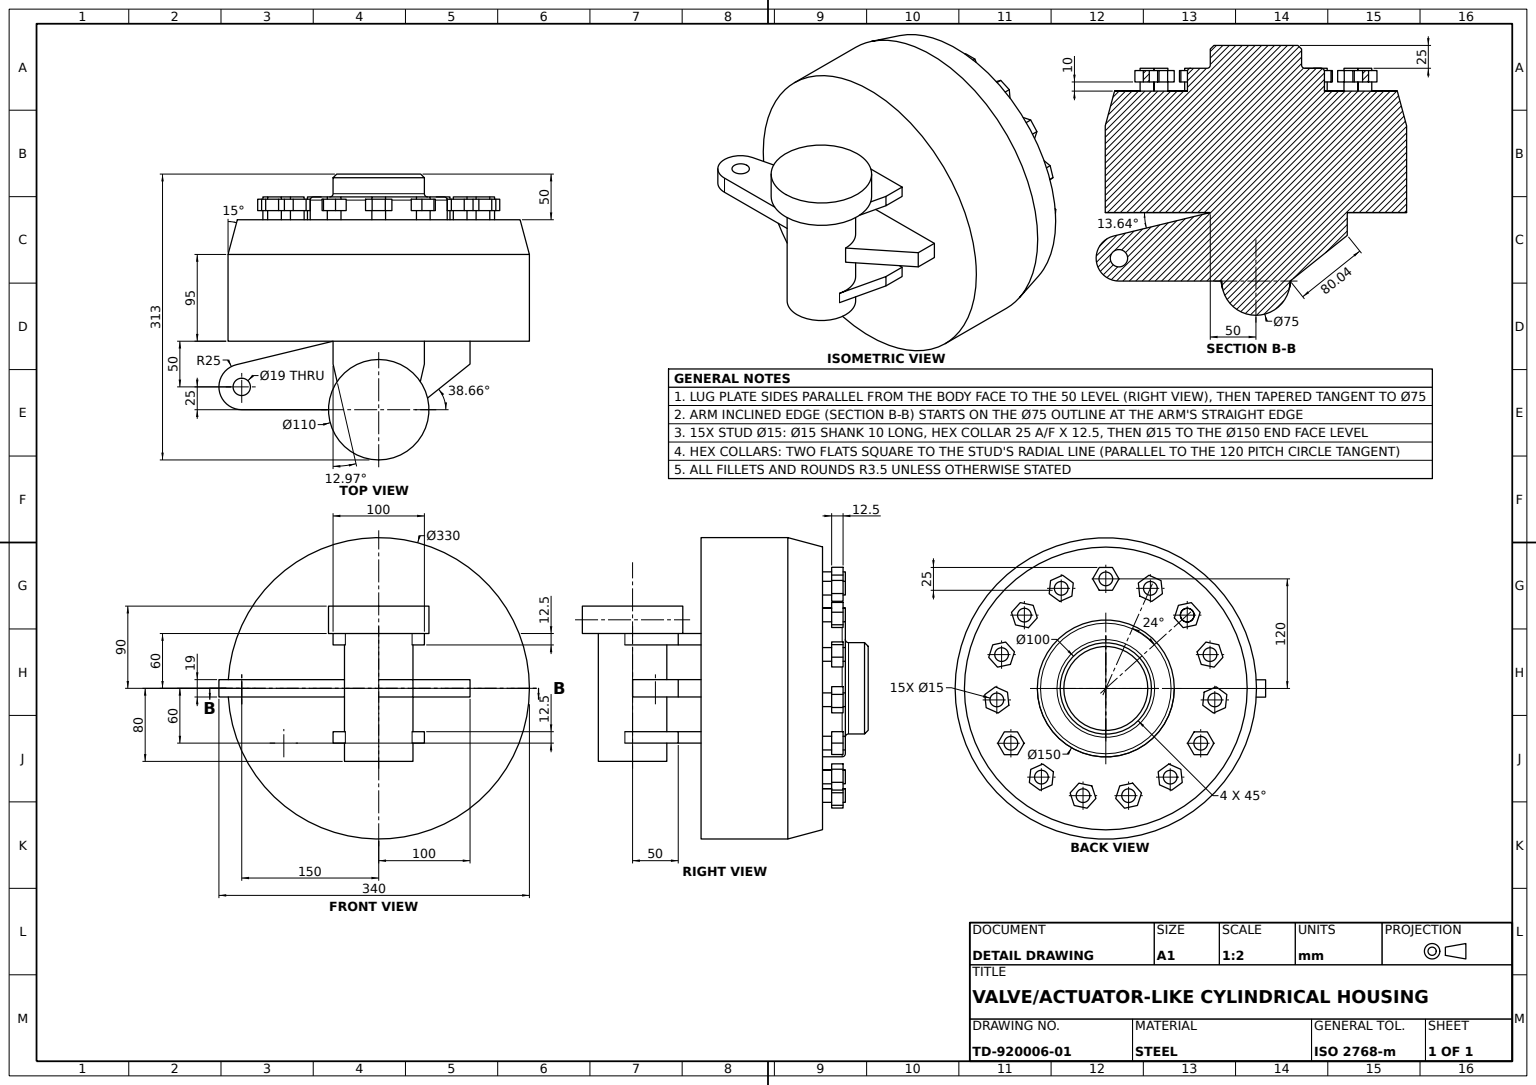
from build123d import *

# Parameters (mm, degrees)
HUB_EDGE_CHAMFER_4MM_SIZE  = 4
HUB_EDGE_FILLET_R3_5_R     = 3.5
SHAFT_BOSS_75_DEPTH        = 90
SHAFT_BOSS_75_DEPTH_BACK   = 80
SHAFT_BOSS_SKETCH_R        = 37.5
LUG_START                  = 60
LUG_12_5MM_DEPTH           = 12.5
BRACKET_ARM_SKETCH_R       = 9.5
BRACKET_ARM_19MM_DEPTH     = 9.5
SHAFT_CAP_SKETCH_R         = 55
SHAFT_CAP_110_DEPTH        = 30
RIM_STUD_SKETCH_R          = 7.5
RIM_STUD_DEPTH             = 25
RIM_START                  = 10
SKETCH9_3_R                = 7.5
RIM_STUD_TAB_DEPTH         = 12.5
RIM_STUD_PATTERN_15X_COUNT = 15


with BuildPart() as part:
    # Hub Profile Sketch → Hub Body Revolve (revolve)
    with BuildSketch(Plane(origin=(0, 0, 0), x_dir=(0, 0, -1), z_dir=(1, 0, 0)), mode=Mode.PRIVATE) as hub_body_revolve_sk:
        Polygon((0, 0), (0, 165), (95, 165), (133, 154.817930688), (133, 75), (158, 75), (158, 50), (183, 50), (183, 0), align=None)
    revolve(hub_body_revolve_sk.sketch.rotate(Axis((0, 0, -183), (0, 0, 1)), 90), axis=Axis((0, 0, -183), (0, 0, 1)))

    # Hub Edge Chamfer 4mm
    hub_edge_chamfer_4mm_edges = [part.edges().sort_by_distance(p)[0] for p in [
        (50, 0, -183),
    ]]
    chamfer(hub_edge_chamfer_4mm_edges, length=HUB_EDGE_CHAMFER_4MM_SIZE)

    # Hub Edge Fillet R3.5
    hub_edge_fillet_r3_5_edges = [part.edges().sort_by_distance(p)[0] for p in [
        (50, 0, -158),
        (75, 0, -158),
    ]]
    fillet(hub_edge_fillet_r3_5_edges, radius=HUB_EDGE_FILLET_R3_5_R)



with BuildPart() as body_2:
    # Shaft Boss Sketch → Shaft Boss _75 (new, two sides: drawn at the far end of the back side and taken through both)
    with BuildSketch(Plane(origin=(0, 0, 0), x_dir=(1, 0, 0), z_dir=(0, 1, 0)).offset(-SHAFT_BOSS_75_DEPTH_BACK)):
        with Locations(Location((0, -75, 0), (0, 0, 270))):
            Circle(SHAFT_BOSS_SKETCH_R)
    extrude(amount=SHAFT_BOSS_75_DEPTH + SHAFT_BOSS_75_DEPTH_BACK)

    # Lug Sketch → Lug 12.5mm (add)
    with BuildSketch(Plane(origin=(0, 0, 0), x_dir=(1, 0, 0), z_dir=(0, 1, 0)).offset(LUG_START)):
        Polygon((36.542960266, -83.417960266), (50, -25), (50, 0), (-50, 0), (-50, -25), (-36.542960266, -83.417960266), align=None)
    lug_12_5mm = extrude(amount=-LUG_12_5MM_DEPTH)

    # Lug Mirror: Lug 12.5mm across plane
    add(lug_12_5mm.mirror(Plane.ZX))


with BuildPart() as part_1:
    add(part.part)

    add(body_2.part)  # Bracket Arm 19mm merges body 2
    # Bracket Arm Sketch → Bracket Arm 19mm (add, symmetric)
    with BuildSketch(Plane(origin=(0, 0, 0), x_dir=(1, 0, 0), z_dir=(0, 1, 0))):
        with BuildLine():
            Line((100, 0), (100, -25))
            Line((100, -25), (37.5, -75))
            ThreePointArc((37.5, -75), (0, -37.5), (-37.5, -75))
            Line((-37.5, -75), (-150, -75))
            ThreePointArc((-150, -75), (-174.822997079, -52.969649142), (-155.897247359, -25.705505282))
            Line((-155.897247359, -25.705505282), (-50, 0))
            Line((-50, 0), (100, 0))
        make_face()
        with Locations(Location((-150, -50, 0), (0, 0, 270))):
            Circle(BRACKET_ARM_SKETCH_R, mode=Mode.SUBTRACT)
    extrude(amount=BRACKET_ARM_19MM_DEPTH, both=True)

    # Shaft Cap Sketch → Shaft Cap _110 (add)
    with BuildSketch(Plane(origin=(0, 60, 0), x_dir=(1, 0, 0), z_dir=(0, 1, 0))):
        with Locations(Location((0, -75, 0), (0, 0, 145.958125966))):
            Circle(SHAFT_CAP_SKETCH_R)
    extrude(amount=SHAFT_CAP_110_DEPTH)

    # Rim Stud Sketch → Rim Stud (add)
    with BuildSketch(Plane(origin=(0, 0, -133), x_dir=(-1, 0, 0), z_dir=(0, 0, -1))):
        with Locations((0, 120)):
            Circle(RIM_STUD_SKETCH_R)
    rim_stud = extrude(amount=RIM_STUD_DEPTH)

    # Sketch9_3 → Rim Stud Tab (add)
    with BuildSketch(Plane(origin=(0, 0, -133), x_dir=(-1, 0, 0), z_dir=(0, 0, -1)).offset(RIM_START)):
        Polygon((7.216878365, 107.5), (14.43375673, 120), (7.216878365, 132.5), (-7.216878365, 132.5), (-14.43375673, 120), (-7.216878365, 107.5), align=None)
        with Locations((0, 120)):
            Circle(SKETCH9_3_R, mode=Mode.SUBTRACT)
    rim_stud_tab = extrude(amount=RIM_STUD_TAB_DEPTH)

    # Rim Stud Pattern 15x: Rim Stud, Rim Stud Tab ×15 about axis
    rim_stud_pattern_15x_axis = Axis((0, 0, 0), (0, 0, 1))
    add([rim_stud.rotate(rim_stud_pattern_15x_axis, i * 360 / RIM_STUD_PATTERN_15X_COUNT) for i in range(1, RIM_STUD_PATTERN_15X_COUNT)])
    add([rim_stud_tab.rotate(rim_stud_pattern_15x_axis, i * 360 / RIM_STUD_PATTERN_15X_COUNT) for i in range(1, RIM_STUD_PATTERN_15X_COUNT)])


solid = part_1.part
